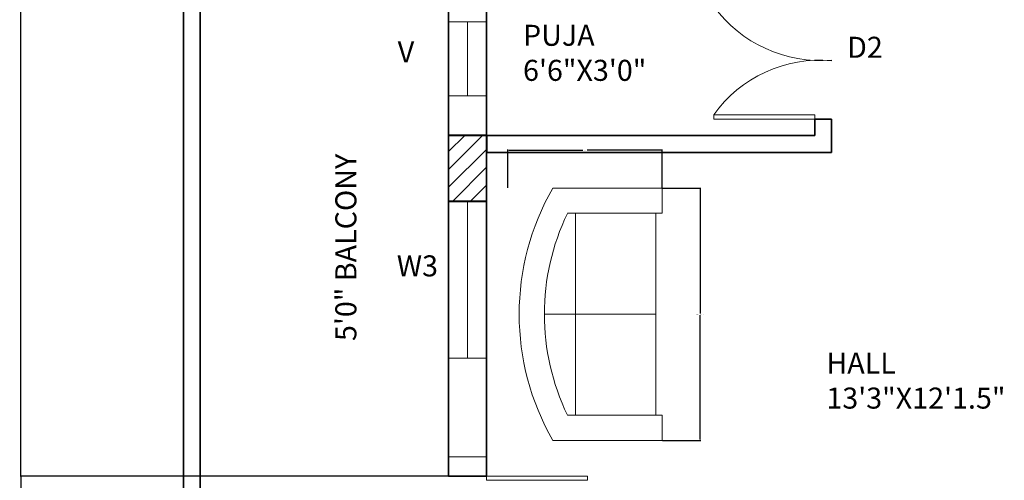
# Model space of a CAD drawing. Units: inches. Extents: x -86 to 2463, y -1058 to 68.
# Tile 11 of 17: x -86 to 148, y -223 to -114. Entities that reach past the tile are written whole.
import ezdxf

# ---------------------------------------------------------------- set-up
doc = ezdxf.new("R2010")
doc.units = ezdxf.units.IN
doc.header["$MEASUREMENT"] = 0
for name, color, linetype, lineweight in [('A-ANNO-DIMS', 2, 'Continuous', 18), ('A-ANNO-TEXT', 7, 'Continuous', 18), ('A-AREA-IDEN', 7, 'Continuous', 18), ('A-COLS', 7, 'Continuous', 40), ('A-COLS-PATT', 252, 'Continuous', 13), ('A-DOOR', 3, 'Continuous', 18), ('A-FURN', 8, 'Continuous', 18), ('A-GLAZ', 4, 'Continuous', 18), ('A-WALL', 7, 'Continuous', 35)]:
    doc.layers.add(name, color=color, linetype=linetype, lineweight=lineweight)
doc.styles.get("Standard").update_dxf_attribs({"font": 'arial.ttf'})
doc.dimstyles.get("Standard").update_dxf_attribs({"dimtxt": 0.18, "dimasz": 0.18, "dimexe": 0.18, "dimexo": 0.0625, "dimgap": 0.09, "dimtad": 0, "dimtih": 1, "dimtoh": 1, "dimdec": 4, "dimzin": 0, "dimdsep": 46, "dimtxsty": 'Standard', "dimcen": 0.09, "dimadec": 0, "dimazin": 0, "dimtfac": 1, "dimtdec": 4, "dimtofl": 0, "dimtmove": 0, "dimatfit": 3, "dimfxl": 1, "dimtolj": 1, "dimtzin": 0, "dimarcsym": 0})

# ---------------------------------------------------------------- blocks, each defined once
blk = doc.blocks.new('Sofa - Roundback Loveseat 5 ft.')
for p, q in [((0, -32.44198), (0, -5.99998)), ((-24, -33.99998), (-24, -11.46958)), ((24.00004, -33.99998), (24.00004, -11.46958)), ((-23.9998, -13.38178), (23.99986, -13.38178)), ((-24, -32.44198), (24.00004, -32.44198))]:
    blk.add_line(p, q)
for points in [[(-24, -33.99998), (-30, -33.99998), (-30, -7.99998)], [(30.00004, -7.99998), (30.00004, -33.99998), (24.00004, -33.99998)]]:
    blk.add_lwpolyline(points)
for centre, radius, start, end in [((0, -60.24998), 60.24998, 60.13715, 119.8628), ((0, -61.38438), 55.38444, 64.32083, 115.6792)]:
    blk.add_arc(centre, radius, start, end)
blk = doc.blocks.new('DOOR-LEAF-24IN')
for p, q in [((0, 0), (0, 24)), ((0, 24), (1, 24)), ((1, 24), (1, 0)), ((1, 0), (0, 0))]:
    blk.add_line(p, q)
blk = doc.blocks.new('*D24')
at = {"layer": 'A-ANNO-DIMS', "color": 0, "lineweight": -2, "transparency": 16777216}
for p, q in [((66.59, -153.6), (75.7, -153.6)), ((75.52, -153.78), (75.52, -183.42)), ((75.52, -213.42), (75.52, -183.79)), ((66.59, -213.6), (75.7, -213.6))]:
    blk.add_line(p, q, dxfattribs=at)
at = {"layer": 'A-ANNO-DIMS', "color": 0, "transparency": 16777216}
for points in [[(75.49, -153.78), (75.55, -153.78), (75.52, -153.6)], [(75.49, -213.42), (75.55, -213.42), (75.52, -213.6)]]:
    blk.add_solid(points, dxfattribs=at)
at = {"layer": 'Defpoints', "color": 0, "transparency": 16777216}
for p in [(66.52, -153.6), (75.52, -153.6), (66.52, -213.6)]:
    blk.add_point(p, dxfattribs=at)
at = {"layer": 'A-ANNO-DIMS', "color": 0, "transparency": 16777216, "insert": (75.52, -183.6), "char_height": 0.18, "attachment_point": 5}
blk.add_mtext('\\A1;LOVESEAT 60 TYP.', dxfattribs=at)
blk = doc.blocks.new('*D25')
at = {"layer": 'A-ANNO-DIMS', "color": 0, "lineweight": -2, "transparency": 16777216}
for p, q in [((29.86, -153.54), (29.86, -144.42)), ((30.04, -144.6), (47.66, -144.6)), ((66.34, -144.6), (48.72, -144.6)), ((66.52, -153.54), (66.52, -144.42))]:
    blk.add_line(p, q, dxfattribs=at)
at = {"layer": 'A-ANNO-DIMS', "color": 0, "transparency": 16777216}
for points in [[(30.04, -144.57), (30.04, -144.63), (29.86, -144.6)], [(66.34, -144.57), (66.34, -144.63), (66.52, -144.6)]]:
    blk.add_solid(points, dxfattribs=at)
at = {"layer": 'Defpoints', "color": 0, "transparency": 16777216}
for p in [(29.86, -144.6), (29.86, -153.6), (66.52, -153.6)]:
    blk.add_point(p, dxfattribs=at)
at = {"layer": 'A-ANNO-DIMS', "color": 0, "transparency": 16777216, "insert": (48.19, -144.6), "char_height": 0.18, "attachment_point": 5}
blk.add_mtext('\\A1;37 TYP.', dxfattribs=at)
blk = doc.blocks.new('*D32')
at = {"layer": 'A-ANNO-DIMS', "color": 0, "lineweight": -2, "transparency": 16777216}
for p, q in [((15.7, 28.9), (-86.02, 28.9)), ((-85.84, 28.72), (-85.84, -96.42)), ((-85.84, -221.92), (-85.84, -96.79)), ((15.7, -222.1), (-86.02, -222.1))]:
    blk.add_line(p, q, dxfattribs=at)
at = {"layer": 'A-ANNO-DIMS', "color": 0, "transparency": 16777216}
for points in [[(-85.87, 28.72), (-85.81, 28.72), (-85.84, 28.9)], [(-85.87, -221.92), (-85.81, -221.92), (-85.84, -222.1)]]:
    blk.add_solid(points, dxfattribs=at)
at = {"layer": 'Defpoints', "color": 0, "transparency": 16777216}
for p in [(-85.84, 28.9), (15.76, 28.9), (15.76, -222.1)]:
    blk.add_point(p, dxfattribs=at)
at = {"layer": 'A-ANNO-DIMS', "color": 0, "transparency": 16777216, "insert": (-85.84, -96.6), "char_height": 0.18, "attachment_point": 5}
blk.add_mtext('\\A1;251', dxfattribs=at)
blk = doc.blocks.new('*D38')
at = {"layer": 'A-ANNO-DIMS', "color": 0, "lineweight": -2, "transparency": 16777216}
for p, q in [((15.7, -222.1), (-86.02, -222.1)), ((-85.84, -222.28), (-85.84, -247.66)), ((-85.84, -273.39), (-85.84, -248.02)), ((15.7, -273.57), (-86.02, -273.57))]:
    blk.add_line(p, q, dxfattribs=at)
at = {"layer": 'A-ANNO-DIMS', "color": 0, "transparency": 16777216}
for points in [[(-85.87, -222.28), (-85.81, -222.28), (-85.84, -222.1)], [(-85.87, -273.39), (-85.81, -273.39), (-85.84, -273.57)]]:
    blk.add_solid(points, dxfattribs=at)
at = {"layer": 'Defpoints', "color": 0, "transparency": 16777216}
for p in [(-85.84, -222.1), (15.76, -222.1), (15.76, -273.57)]:
    blk.add_point(p, dxfattribs=at)
at = {"layer": 'A-ANNO-DIMS', "color": 0, "transparency": 16777216, "insert": (-85.84, -247.84), "char_height": 0.18, "attachment_point": 5}
blk.add_mtext('\\A1;51.47', dxfattribs=at)

msp = doc.modelspace()

# ---------------------------------------------------------------- hatches: boundary and pattern name
at = {"layer": 'A-COLS-PATT'}
h = msp.add_hatch(dxfattribs=at)
h.set_pattern_fill('ANSI31', color=256, scale=24)
h.set_pattern_definition([(45, (-1015.1314, -586.0864), (-2.1213203, 2.1213203), [])])
h.paths.add_polyline_path([(24.761, -294.104), (24.761, -284.978), (15.761, -284.978), (15.761, -303.104), (24.761, -303.104)])
h.paths.add_polyline_path([(199.1, -294.104), (183.761, -294.104), (183.761, -303.104), (199.1, -303.104)])
h.paths.add_polyline_path([(386.761, -294.104), (377.761, -294.104), (369.914, -294.104), (369.914, -303.104), (377.846, -303.104), (386.761, -303.104)])
h.paths.add_polyline_path([(386.761, -145.104), (386.761, -141.104), (377.761, -141.104), (377.761, -145.104), (377.761, -154.61), (386.761, -154.61)])
h.paths.add_polyline_path([(386.761, -154.61), (377.761, -154.61), (377.761, -162.891), (386.761, -162.891)])
h.paths.add_polyline_path([(24.761, -145.104), (24.761, -141.104), (15.761, -141.104), (15.761, -156.678), (24.761, -156.678)])
h.paths.add_polyline_path([(-38.239, 28.896), (-47.239, 28.896), (-47.239, 19.896), (-47.239, 12.652), (-38.239, 12.652), (-38.239, 19.896)])
h.paths.add_polyline_path([(24.761, 28.896), (15.761, 28.896), (15.761, 19.896), (15.761, 12.545), (24.761, 12.545), (24.761, 19.896)])
h.paths.add_polyline_path([(183.507, 19.896), (161.036, 19.896), (161.036, 17.001), (183.507, 17.001)])
h.paths.add_polyline_path([(183.507, 28.896), (161.036, 28.896), (161.036, 19.896), (183.507, 19.896)])
h.paths.add_polyline_path([(386.761, 28.896), (373.166, 28.896), (373.166, 19.896), (377.761, 19.896), (386.761, 19.896)])

# ---------------------------------------------------------------- linework, layer by layer
at = {"layer": 'A-COLS'}
for p, q in [((24.761, -141.104), (15.761, -141.104)), ((24.761, -141.104), (24.761, -145.104)), ((15.761, -156.678), (24.761, -156.678))]:
    msp.add_line(p, q, dxfattribs=at)
at = {"layer": 'A-DOOR'}
msp.add_line((106.761, -123.179), (106.761, -123.31), dxfattribs=at)
for centre, radius, start, end in [((104.302, -91.48), 31.795, 216.55167, 274.43502), ((103.928, -154.006), 30.827, 84.72726, 144.72726)]:
    msp.add_arc(centre, radius, start, end, dxfattribs=at)
at = {"layer": 'A-GLAZ'}
for p, q in [((15.761, -114.059), (24.761, -114.059)), ((20.261, -114.059), (20.261, -131.665)), ((15.761, -131.665), (24.761, -131.665)), ((20.261, -156.678), (20.261, -194.059)), ((15.761, -194.059), (24.761, -194.059)), ((15.761, -217.507), (24.761, -217.507))]:
    msp.add_line(p, q, dxfattribs=at)
at = {"layer": 'A-WALL'}
for p, q in [((-47.239, -141.104), (-47.239, 19.896)), ((15.761, -141.104), (15.761, 19.896)), ((-43.239, -141.104), (-43.239, -61.104)), ((24.761, -105.104), (24.761, -141.104)), ((102.761, -137.204), (106.761, -137.204)), ((102.761, -137.204), (102.761, -141.104)), ((106.761, -137.204), (106.761, -141.104)), ((-47.239, -141.104), (-47.239, -701.604)), ((-43.239, -141.104), (-43.239, -697.604)), ((15.761, -141.104), (15.761, -222.104)), ((102.761, -141.104), (24.761, -141.104)), ((106.761, -141.104), (106.761, -145.104)), ((106.761, -145.104), (24.761, -145.104)), ((24.761, -145.104), (24.761, -222.104)), ((15.761, -222.104), (24.761, -222.104))]:
    msp.add_line(p, q, dxfattribs=at)

# ---------------------------------------------------------------- block references
at = {"layer": 'A-DOOR'}
for p, rotation in [((78.761, -136.204), 270.0000000000002), ((48.761, -223.104), 90.00000000000007)]:
    msp.add_blockref('DOOR-LEAF-24IN', p, dxfattribs=dict(at, rotation=rotation))
at = {"layer": 'A-FURN', "rotation": 90}
msp.add_blockref('Sofa - Roundback Loveseat 5 ft.', (32.525, -183.604), dxfattribs=at)

# ---------------------------------------------------------------- texts
at = {"layer": 'A-ANNO-TEXT', "char_height": 5, "attachment_point": 1}
for s, width, insert in [('V', 5.92026, (3.667, -118.725)), ('D2', 14.145, (110.446, -117.613)), ('W3', 12.29818, (3.463, -169.604))]:
    msp.add_mtext_dynamic_manual_height_columns(s, width=width, gutter_width=25, heights=[0], dxfattribs=dict(at, insert=insert))
at = {"layer": 'A-AREA-IDEN', "char_height": 5, "attachment_point": 1}
for s, width, insert in [('PUJA\\P6\'6"X3\'0"', 37.67583, (33.441, -114.761)), ('HALL\\P13\'3"X12\'1.5"', 75.18459, (105.51, -192.715))]:
    msp.add_mtext_dynamic_manual_height_columns(s, width=width, gutter_width=25, heights=[0], dxfattribs=dict(at, insert=insert))
at = {"layer": 'A-AREA-IDEN', "insert": (-11.148, -189.971), "char_height": 5, "attachment_point": 1, "rotation": 90}
msp.add_mtext_dynamic_manual_height_columns('5\'0" BALCONY', width=106.5034, gutter_width=25, heights=[0], dxfattribs=at)

# ---------------------------------------------------------------- dimensions: what is measured, and where the dimension line sits
at = {"layer": 'A-ANNO-DIMS'}
for base, p1, p2, override, picture, middle in [((-85.839, 28.896), (15.761, -222.104), (15.761, 28.896), {"dimdec": 0, "dimlfac": 1, "dimrnd": 0, "dimzin": 0, "dimdsep": 46, "dimlunit": 2}, '*D32', (-85.839, -96.604)), ((-85.839, -222.104), (15.761, -273.574), (15.761, -222.104), {"dimdec": 2, "dimlfac": 1, "dimrnd": 0, "dimzin": 0, "dimdsep": 46, "dimlunit": 2}, '*D38', (-85.839, -247.839))]:
    dim = msp.add_linear_dim(base=base, p1=p1, p2=p2, angle=90, dimstyle='Standard', override=override, dxfattribs=at)
    dim.commit()
    dim.dimension.update_dxf_attribs({"geometry": picture, "text_midpoint": middle})
for base, p1, p2, angle, text, picture, middle in [((29.858, -144.604), (66.525, -153.604), (29.858, -153.604), 180, '<> TYP.', '*D25', (48.192, -144.604)), ((75.525, -153.604), (66.525, -213.604), (66.525, -153.604), 90, 'LOVESEAT <> TYP.', '*D24', (75.525, -183.604))]:
    dim = msp.add_linear_dim(base=base, p1=p1, p2=p2, angle=angle, text=text, dimstyle='Standard', override={"dimdec": 0, "dimlfac": 1, "dimrnd": 0, "dimzin": 0, "dimdsep": 46, "dimlunit": 2}, dxfattribs=at)
    dim.commit()
    dim.dimension.update_dxf_attribs({"geometry": picture, "text_midpoint": middle})

doc.saveas('drawing.dxf')
